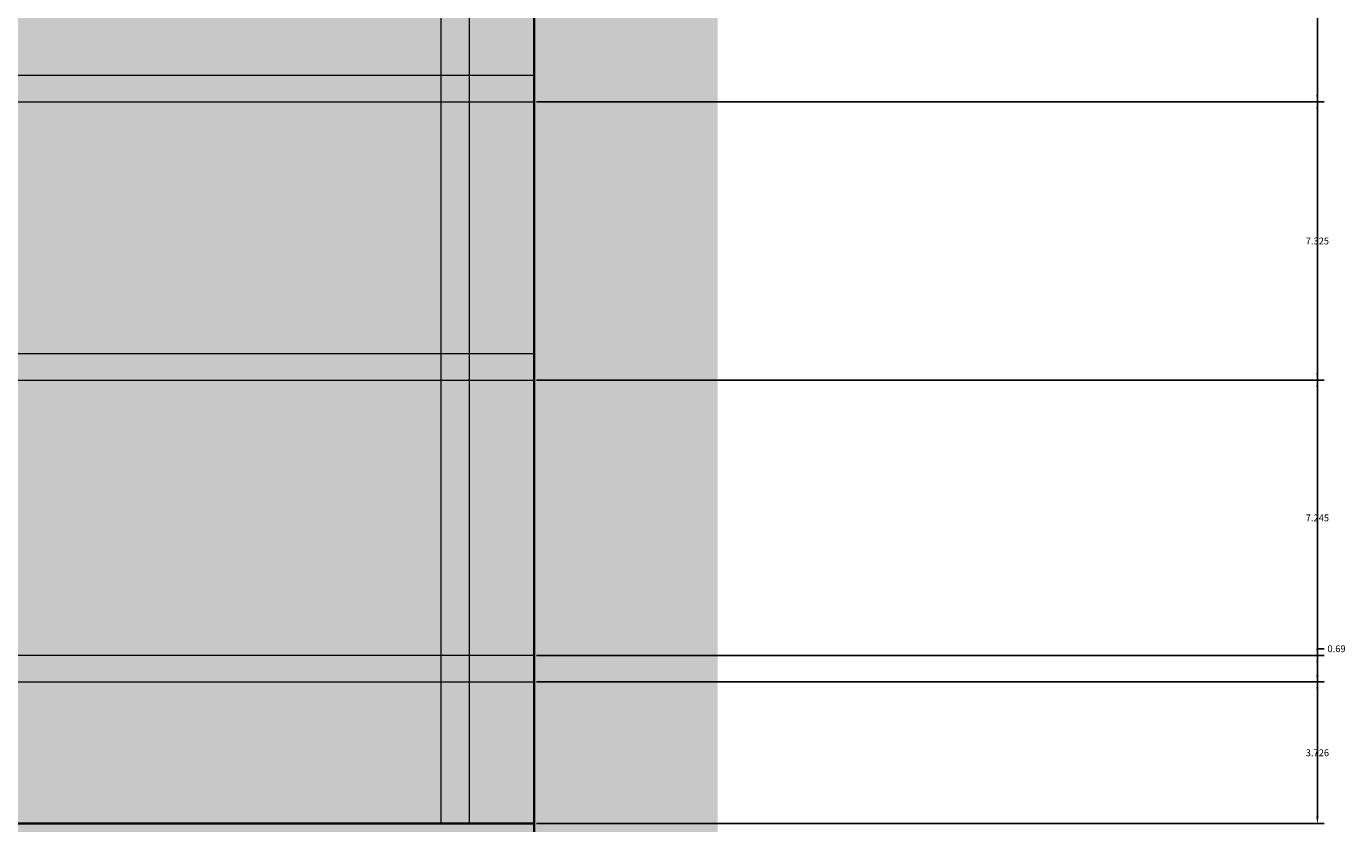
# Model space of a CAD drawing. Units: feet. Extents: x 2695 to 2912, y 795 to 1139.
# Tile 59 of 83: x 2877 to 2912, y 937 to 958. Entities that reach past the tile are written whole.
import ezdxf

# ---------------------------------------------------------------- set-up
doc = ezdxf.new("R2010")
doc.units = ezdxf.units.FT
for name, color, linetype, lineweight in [('A-ANNO-DIMS', 2, 'Continuous', 18), ('A-ELEV', 7, 'Continuous', 35), ('A-ELEV-PATT', 252, 'Continuous', 13), ('A-ELEV-RAIL', 8, 'Continuous', 18)]:
    doc.layers.add(name, color=color, linetype=linetype, lineweight=lineweight)
doc.styles.get("Standard").update_dxf_attribs({"font": 'arial.ttf'})
doc.dimstyles.get("Standard").update_dxf_attribs({"dimtxt": 0.18, "dimasz": 0.18, "dimexe": 0.18, "dimexo": 0.0625, "dimgap": 0.09, "dimtad": 0, "dimtih": 1, "dimtoh": 1, "dimdec": 1, "dimzin": 0, "dimdsep": 46, "dimlunit": 3, "dimtxsty": 'Standard', "dimcen": 0.09, "dimadec": 0, "dimazin": 0, "dimtfac": 1, "dimtdec": 1, "dimtofl": 0, "dimtmove": 0, "dimatfit": 3, "dimfxl": 1, "dimtolj": 1, "dimtzin": 0, "dimarcsym": 0})

# ---------------------------------------------------------------- blocks, each defined once
blk = doc.blocks.new('*D17')
at = {"layer": 'A-ANNO-DIMS', "color": 0, "lineweight": -2, "transparency": 16777216}
for p, q in [((2843.637, 1020.824), (2911.424, 1020.824)), ((2911.244, 1020.644), (2911.244, 979.059)), ((2911.244, 937.111), (2911.244, 978.695)), ((2890.699, 936.931), (2911.424, 936.931))]:
    blk.add_line(p, q, dxfattribs=at)
at = {"layer": 'A-ANNO-DIMS', "color": 0, "transparency": 16777216}
for points in [[(2911.214, 1020.644), (2911.274, 1020.644), (2911.244, 1020.824)], [(2911.214, 937.111), (2911.274, 937.111), (2911.244, 936.931)]]:
    blk.add_solid(points, dxfattribs=at)
at = {"layer": 'Defpoints', "color": 0, "transparency": 16777216}
for p in [(2843.575, 1020.824), (2911.244, 1020.824), (2890.636, 936.931)]:
    blk.add_point(p, dxfattribs=at)
at = {"layer": 'A-ANNO-DIMS', "color": 0, "transparency": 16777216, "insert": (2911.244, 978.877), "char_height": 0.18, "attachment_point": 5}
blk.add_mtext('\\A1;83.9', dxfattribs=at)
blk = doc.blocks.new('*D53')
at = {"layer": 'A-ANNO-DIMS', "color": 0, "lineweight": -2, "transparency": 16777216}
for p, q in [((2890.699, 940.657), (2911.424, 940.657)), ((2911.244, 940.477), (2911.244, 938.976)), ((2911.244, 937.111), (2911.244, 938.612)), ((2890.699, 936.931), (2911.424, 936.931))]:
    blk.add_line(p, q, dxfattribs=at)
at = {"layer": 'A-ANNO-DIMS', "color": 0, "transparency": 16777216}
for points in [[(2911.214, 940.477), (2911.274, 940.477), (2911.244, 940.657)], [(2911.214, 937.111), (2911.274, 937.111), (2911.244, 936.931)]]:
    blk.add_solid(points, dxfattribs=at)
at = {"layer": 'Defpoints', "color": 0, "transparency": 16777216}
for p in [(2890.636, 940.657), (2911.244, 940.657), (2890.636, 936.931)]:
    blk.add_point(p, dxfattribs=at)
at = {"layer": 'A-ANNO-DIMS', "color": 0, "transparency": 16777216, "insert": (2911.244, 938.794), "char_height": 0.18, "attachment_point": 5}
blk.add_mtext('\\A1;3.726', dxfattribs=at)
blk = doc.blocks.new('*D54')
at = {"layer": 'A-ANNO-DIMS', "color": 0, "lineweight": -2, "transparency": 16777216}
for p, q in [((2890.699, 941.351), (2911.424, 941.351)), ((2911.244, 941.351), (2911.244, 941.531)), ((2911.244, 941.531), (2911.424, 941.531)), ((2911.244, 940.837), (2911.244, 941.171)), ((2890.699, 940.657), (2911.424, 940.657))]:
    blk.add_line(p, q, dxfattribs=at)
at = {"layer": 'A-ANNO-DIMS', "color": 0, "transparency": 16777216}
for points in [[(2911.214, 941.171), (2911.274, 941.171), (2911.244, 941.351)], [(2911.214, 940.837), (2911.274, 940.837), (2911.244, 940.657)]]:
    blk.add_solid(points, dxfattribs=at)
at = {"layer": 'Defpoints', "color": 0, "transparency": 16777216}
for p in [(2890.636, 941.351), (2911.244, 941.351), (2890.636, 940.657)]:
    blk.add_point(p, dxfattribs=at)
at = {"layer": 'A-ANNO-DIMS', "color": 0, "transparency": 16777216, "insert": (2911.748, 941.531), "char_height": 0.18, "attachment_point": 5}
blk.add_mtext('\\A1;0.69', dxfattribs=at)
blk = doc.blocks.new('*D55')
at = {"layer": 'A-ANNO-DIMS', "color": 0, "lineweight": -2, "transparency": 16777216}
for p, q in [((2890.699, 948.595), (2911.424, 948.595)), ((2911.244, 948.415), (2911.244, 945.155)), ((2911.244, 941.531), (2911.244, 944.791)), ((2890.699, 941.351), (2911.424, 941.351))]:
    blk.add_line(p, q, dxfattribs=at)
at = {"layer": 'A-ANNO-DIMS', "color": 0, "transparency": 16777216}
for points in [[(2911.214, 948.415), (2911.274, 948.415), (2911.244, 948.595)], [(2911.214, 941.531), (2911.274, 941.531), (2911.244, 941.351)]]:
    blk.add_solid(points, dxfattribs=at)
at = {"layer": 'Defpoints', "color": 0, "transparency": 16777216}
for p in [(2890.636, 948.595), (2911.244, 948.595), (2890.636, 941.351)]:
    blk.add_point(p, dxfattribs=at)
at = {"layer": 'A-ANNO-DIMS', "color": 0, "transparency": 16777216, "insert": (2911.244, 944.973), "char_height": 0.18, "attachment_point": 5}
blk.add_mtext('\\A1;7.245', dxfattribs=at)
blk = doc.blocks.new('*D56')
at = {"layer": 'A-ANNO-DIMS', "color": 0, "lineweight": -2, "transparency": 16777216}
for p, q in [((2890.699, 955.92), (2911.424, 955.92)), ((2911.244, 955.74), (2911.244, 952.44)), ((2911.244, 948.775), (2911.244, 952.076)), ((2890.699, 948.595), (2911.424, 948.595))]:
    blk.add_line(p, q, dxfattribs=at)
at = {"layer": 'A-ANNO-DIMS', "color": 0, "transparency": 16777216}
for points in [[(2911.214, 955.74), (2911.274, 955.74), (2911.244, 955.92)], [(2911.214, 948.775), (2911.274, 948.775), (2911.244, 948.595)]]:
    blk.add_solid(points, dxfattribs=at)
at = {"layer": 'Defpoints', "color": 0, "transparency": 16777216}
for p in [(2890.636, 955.92), (2911.244, 955.92), (2890.636, 948.595)]:
    blk.add_point(p, dxfattribs=at)
at = {"layer": 'A-ANNO-DIMS', "color": 0, "transparency": 16777216, "insert": (2911.244, 952.258), "char_height": 0.18, "attachment_point": 5}
blk.add_mtext('\\A1;7.325', dxfattribs=at)
blk = doc.blocks.new('*D57')
at = {"layer": 'A-ANNO-DIMS', "color": 0, "lineweight": -2, "transparency": 16777216}
for p, q in [((2890.699, 964.133), (2911.424, 964.133)), ((2911.244, 963.953), (2911.244, 960.208)), ((2911.244, 956.1), (2911.244, 959.845)), ((2890.699, 955.92), (2911.424, 955.92))]:
    blk.add_line(p, q, dxfattribs=at)
at = {"layer": 'A-ANNO-DIMS', "color": 0, "transparency": 16777216}
for points in [[(2911.214, 963.953), (2911.274, 963.953), (2911.244, 964.133)], [(2911.214, 956.1), (2911.274, 956.1), (2911.244, 955.92)]]:
    blk.add_solid(points, dxfattribs=at)
at = {"layer": 'Defpoints', "color": 0, "transparency": 16777216}
for p in [(2890.636, 964.133), (2911.244, 964.133), (2890.636, 955.92)]:
    blk.add_point(p, dxfattribs=at)
at = {"layer": 'A-ANNO-DIMS', "color": 0, "transparency": 16777216, "insert": (2911.244, 960.027), "char_height": 0.18, "attachment_point": 5}
blk.add_mtext('\\A1;8.213', dxfattribs=at)

msp = doc.modelspace()

# ---------------------------------------------------------------- hatches: boundary and pattern name
at = {"layer": 'A-ELEV-PATT'}
h = msp.add_hatch(color=256, dxfattribs=at)
h.set_gradient(color1=(255, 255, 255), tint=1)
h.paths.add_polyline_path([(2770.6361, 1122.9306), (2710.6361, 1122.9306), (2710.6361, 1118.4096), (2770.6361, 1118.4096)])
h.paths.add_polyline_path([(2890.6361, 1107.8588), (2770.6361, 1107.8588), (2770.6361, 1103.3378), (2890.6361, 1103.3378)])
h.paths.add_polyline_path([(2890.6361, 1062.9306), (2710.6361, 1062.9306), (2710.6361, 1056.9306), (2710.6361, 936.9306), (2710.6361, 924.3105), (2716.5358, 924.3105), (2890.6361, 924.3105), (2890.6361, 936.9306), (2715.8852, 936.9306), (2715.8852, 1050.3105), (2890.6361, 1050.3105)])
h.paths.add_polyline_path([(2716.5358, 924.3105), (2710.6361, 924.3105), (2710.6361, 810.9306), (2716.5358, 810.9306)])
h = msp.add_hatch(color=256, dxfattribs=at)
h.set_gradient(color1=(147, 149, 152), color2=(147, 149, 152), tint=1)
h.paths.add_polyline_path([(2770.6361, 1118.4096), (2710.6361, 1118.4096), (2710.6361, 1062.9306), (2770.6361, 1062.9306)])
h.paths.add_polyline_path([(2890.6361, 1103.3378), (2770.6361, 1103.3378), (2770.6361, 1062.9306), (2890.6361, 1062.9306)])
h.paths.add_polyline_path([(2730.7081, 1048.1052), (2755.1125, 1048.1052), (2755.1125, 936.9306), (2770.6361, 936.9306), (2770.6361, 1050.3105), (2715.8852, 1050.3105), (2715.8852, 936.9306), (2730.7081, 936.9306)])
h.paths.add_polyline_path([(2890.6361, 1050.3105), (2770.6361, 1050.3105), (2770.6361, 971.9673), (2778.0341, 971.9673), (2778.0341, 1020.8235), (2843.575, 1020.8235), (2843.575, 971.9673), (2890.6361, 971.9673)])
h.paths.add_polyline_path([(2888.1882, 970.7156), (2843.575, 970.7156), (2843.575, 964.8267), (2888.1882, 964.8267)])
h.paths.add_polyline_path([(2888.1882, 964.1328), (2843.575, 964.1328), (2843.575, 956.614), (2888.1882, 956.614)])
h.paths.add_polyline_path([(2888.1882, 955.9202), (2843.575, 955.9202), (2843.575, 949.2892), (2888.1882, 949.2892)])
h.paths.add_polyline_path([(2888.1882, 948.5954), (2843.575, 948.5954), (2843.575, 941.3507), (2888.1882, 941.3507)])
h.paths.add_polyline_path([(2888.1882, 940.6569), (2843.575, 940.6569), (2843.575, 936.9306), (2888.1882, 936.9306)])
h.paths.add_polyline_path([(2890.6361, 970.7156), (2888.9368, 970.7156), (2888.9368, 964.8267), (2890.6361, 964.8267)])
h.paths.add_polyline_path([(2890.6361, 964.1328), (2888.9368, 964.1328), (2888.9368, 956.614), (2890.6361, 956.614)])
h.paths.add_polyline_path([(2890.6361, 955.9202), (2888.9368, 955.9202), (2888.9368, 949.2892), (2890.6361, 949.2892)])
h.paths.add_polyline_path([(2890.6361, 940.6569), (2888.9368, 940.6569), (2888.9368, 936.9306), (2890.6361, 936.9306)])
h.paths.add_polyline_path([(2890.6361, 948.5954), (2888.9368, 948.5954), (2888.9368, 941.3507), (2890.6361, 941.3507)])
h.paths.add_polyline_path([(2772.5216, 970.7156), (2770.6361, 970.7156), (2770.6361, 964.8267), (2772.5216, 964.8267)])
h.paths.add_polyline_path([(2772.5216, 964.1328), (2770.6361, 964.1328), (2770.6361, 956.614), (2772.5216, 956.614)])
h.paths.add_polyline_path([(2772.5216, 955.9202), (2770.6361, 955.9202), (2770.6361, 949.2892), (2772.5216, 949.2892)])
h.paths.add_polyline_path([(2772.5216, 948.5954), (2770.6361, 948.5954), (2770.6361, 941.3507), (2772.5216, 941.3507)])
h.paths.add_polyline_path([(2772.5216, 940.6569), (2770.6361, 940.6569), (2770.6361, 936.9306), (2772.5216, 936.9306)])
h.paths.add_polyline_path([(2778.0341, 940.6569), (2773.2702, 940.6569), (2773.2702, 936.9306), (2778.0341, 936.9306)])
h.paths.add_polyline_path([(2778.0341, 970.7156), (2773.2702, 970.7156), (2773.2702, 964.8267), (2778.0341, 964.8267)])
h.paths.add_polyline_path([(2778.0341, 964.1328), (2773.2702, 964.1328), (2773.2702, 956.614), (2778.0341, 956.614)])
h.paths.add_polyline_path([(2778.0341, 955.9202), (2773.2702, 955.9202), (2773.2702, 949.2892), (2778.0341, 949.2892)])
h.paths.add_polyline_path([(2778.0341, 948.5954), (2773.2702, 948.5954), (2773.2702, 941.3507), (2778.0341, 941.3507)])
h.paths.add_polyline_path([(2810.0407, 940.6569), (2780.0341, 940.6569), (2780.0341, 936.9306), (2810.0407, 936.9306)])
h.paths.add_polyline_path([(2890.6361, 924.3105), (2770.6361, 924.3105), (2770.6361, 810.9306), (2773.5029, 810.9306), (2773.5029, 905.5143), (2805.9398, 905.5143), (2838.3767, 905.5143), (2838.3767, 810.9306), (2890.6361, 810.9306)])
h = msp.add_hatch(color=256, dxfattribs=at)
h.set_gradient(color1=(255, 255, 255), tint=1)
h.paths.add_polyline_path([(2895.4694, 1107.8588), (2890.6361, 1107.8588), (2890.6361, 810.9306), (2895.4694, 810.9306)])
h = msp.add_hatch(color=256, dxfattribs=at)
h.set_gradient(color1=(255, 255, 255), tint=1)
h.paths.add_polyline_path([(2890.6361, 1050.3105), (2881.9484, 1050.3105), (2881.9484, 971.9673), (2890.6361, 971.9673)])
h.paths.add_polyline_path([(2888.1882, 970.7156), (2881.9484, 970.7156), (2881.9484, 964.8267), (2888.1882, 964.8267)])
h.paths.add_polyline_path([(2890.6361, 970.7156), (2888.9368, 970.7156), (2888.9368, 964.8267), (2890.6361, 964.8267)])
h.paths.add_polyline_path([(2888.1882, 964.1328), (2881.9484, 964.1328), (2881.9484, 956.614), (2888.1882, 956.614)])
h.paths.add_polyline_path([(2890.6361, 964.1328), (2888.9368, 964.1328), (2888.9368, 956.614), (2890.6361, 956.614)])
h.paths.add_polyline_path([(2888.1882, 955.9202), (2881.9484, 955.9202), (2881.9484, 949.2892), (2888.1882, 949.2892)])
h.paths.add_polyline_path([(2890.6361, 955.9202), (2888.9368, 955.9202), (2888.9368, 949.2892), (2890.6361, 949.2892)])
h.paths.add_polyline_path([(2888.1882, 948.5954), (2881.9484, 948.5954), (2881.9484, 941.3507), (2888.1882, 941.3507)])
h.paths.add_polyline_path([(2890.6361, 948.5954), (2888.9368, 948.5954), (2888.9368, 941.3507), (2890.6361, 941.3507)])
h.paths.add_polyline_path([(2888.1882, 940.6569), (2881.9484, 940.6569), (2881.9484, 936.9306), (2888.1882, 936.9306)])
h = msp.add_hatch(color=256, dxfattribs=at)
h.set_gradient(color2=(0, 0, 0), tint=1)
h.paths.add_polyline_path([(2772.5216, 971.9673), (2770.6361, 971.9673), (2770.6361, 970.7156), (2772.5216, 970.7156)])
h.paths.add_polyline_path([(2773.2702, 971.9673), (2772.5216, 971.9673), (2772.5216, 970.7156), (2773.2702, 970.7156)])
h.paths.add_polyline_path([(2778.0341, 971.9673), (2773.2702, 971.9673), (2773.2702, 970.7156), (2778.0341, 970.7156)])
h.paths.add_polyline_path([(2780.0341, 971.9673), (2778.0341, 971.9673), (2778.0341, 970.7156), (2780.0341, 970.7156)])
h.paths.add_polyline_path([(2841.575, 971.9673), (2780.0341, 971.9673), (2780.0341, 970.7156), (2841.575, 970.7156)])
h.paths.add_polyline_path([(2843.575, 971.9673), (2841.575, 971.9673), (2841.575, 970.7156), (2843.575, 970.7156)])
h.paths.add_polyline_path([(2888.1882, 971.9673), (2843.575, 971.9673), (2843.575, 970.7156), (2888.1882, 970.7156)])
h.paths.add_polyline_path([(2888.9368, 971.9673), (2888.1882, 971.9673), (2888.1882, 970.7156), (2888.9368, 970.7156)], flags=17)
h.paths.add_polyline_path([(2890.6361, 971.9673), (2888.9368, 971.9673), (2888.9368, 970.7156), (2890.6361, 970.7156)])
h.paths.add_polyline_path([(2888.9368, 971.9673), (2888.1882, 971.9673), (2888.1882, 964.8267), (2888.9368, 964.8267)])
h.paths.add_polyline_path([(2888.9368, 964.8267), (2888.1882, 964.8267), (2888.1882, 964.1328), (2888.9368, 964.1328)])
h.paths.add_polyline_path([(2890.6361, 964.8267), (2888.9368, 964.8267), (2888.9368, 964.1328), (2890.6361, 964.1328)])
h.paths.add_polyline_path([(2888.1882, 964.8267), (2770.6361, 964.8267), (2770.6361, 964.1328), (2888.1882, 964.1328)])
h.paths.add_polyline_path([(2888.9368, 964.1328), (2888.1882, 964.1328), (2888.1882, 936.9306), (2888.9368, 936.9306)])
h.paths.add_polyline_path([(2890.6361, 956.614), (2888.9368, 956.614), (2888.9368, 955.9202), (2890.6361, 955.9202)])
h.paths.add_polyline_path([(2888.1882, 956.614), (2770.6361, 956.614), (2770.6361, 955.9202), (2888.1882, 955.9202)])
h.paths.add_polyline_path([(2890.6361, 949.2892), (2888.9368, 949.2892), (2888.9368, 948.5954), (2890.6361, 948.5954)])
h.paths.add_polyline_path([(2888.1882, 949.2892), (2770.6361, 949.2892), (2770.6361, 948.5954), (2888.1882, 948.5954)])
h.paths.add_polyline_path([(2890.6361, 941.3507), (2888.9368, 941.3507), (2888.9368, 940.6569), (2890.6361, 940.6569)])
h.paths.add_polyline_path([(2888.1882, 941.3507), (2770.6361, 941.3507), (2770.6361, 940.6569), (2888.1882, 940.6569)])
h.paths.add_polyline_path([(2773.2702, 970.7156), (2772.5216, 970.7156), (2772.5216, 964.8267), (2773.2702, 964.8267)])
h.paths.add_polyline_path([(2773.2702, 964.1328), (2772.5216, 964.1328), (2772.5216, 956.614), (2773.2702, 956.614)])
h.paths.add_polyline_path([(2773.2702, 955.9202), (2772.5216, 955.9202), (2772.5216, 936.9306), (2773.2702, 936.9306)])
h.paths.add_polyline_path([(2810.7893, 970.7156), (2810.0407, 970.7156), (2810.0407, 964.8267), (2810.7893, 964.8267)], flags=17)
h.paths.add_polyline_path([(2810.7893, 964.1328), (2810.0407, 964.1328), (2810.0407, 956.614), (2810.7893, 956.614)], flags=17)
h.paths.add_polyline_path([(2810.7893, 955.9202), (2810.0407, 955.9202), (2810.0407, 949.2892), (2810.7893, 949.2892)], flags=17)
h.paths.add_polyline_path([(2810.7893, 971.9673), (2810.0407, 971.9673), (2810.0407, 941.3507), (2810.7893, 941.3507)])
h.paths.add_polyline_path([(2810.7893, 940.6569), (2810.0407, 940.6569), (2810.0407, 936.9306), (2810.7893, 936.9306)])
h.paths.add_polyline_path([(2780.0341, 1018.8235), (2841.575, 1018.8235), (2841.575, 971.9673), (2843.575, 971.9673), (2843.575, 1020.8235), (2778.0341, 1020.8235), (2778.0341, 971.9673), (2780.0341, 971.9673)])
h.paths.add_polyline_path([(2780.0341, 970.7156), (2778.0341, 970.7156), (2778.0341, 964.8267), (2780.0341, 964.8267)])
h.paths.add_polyline_path([(2780.0341, 964.1328), (2778.0341, 964.1328), (2778.0341, 956.614), (2780.0341, 956.614)])
h.paths.add_polyline_path([(2780.0341, 955.9202), (2778.0341, 955.9202), (2778.0341, 949.2892), (2780.0341, 949.2892)])
h.paths.add_polyline_path([(2780.0341, 948.5954), (2778.0341, 948.5954), (2778.0341, 941.3507), (2780.0341, 941.3507)])
h.paths.add_polyline_path([(2780.0341, 940.6569), (2778.0341, 940.6569), (2778.0341, 936.9306), (2780.0341, 936.9306)])
h.paths.add_polyline_path([(2843.575, 940.6569), (2841.575, 940.6569), (2841.575, 936.9306), (2843.575, 936.9306)])
h.paths.add_polyline_path([(2843.575, 948.5954), (2841.575, 948.5954), (2841.575, 941.3507), (2843.575, 941.3507)])
h.paths.add_polyline_path([(2843.575, 970.7156), (2841.575, 970.7156), (2841.575, 964.8267), (2843.575, 964.8267)])
h.paths.add_polyline_path([(2843.575, 964.1328), (2841.575, 964.1328), (2841.575, 956.614), (2843.575, 956.614)])
h.paths.add_polyline_path([(2843.575, 955.9202), (2841.575, 955.9202), (2841.575, 949.2892), (2843.575, 949.2892)])
h.paths.add_polyline_path([(2805.0538, 874.1057), (2803.9681, 874.1057), (2803.9681, 846.2857), (2805.0538, 846.2857)])
h.paths.add_polyline_path([(2758.1515, 902.577), (2724.1893, 902.577), (2724.1893, 874.8571), (2758.1515, 874.8571)])
h.paths.add_polyline_path([(2726.1893, 900.577), (2756.1515, 900.577), (2756.1515, 876.8571), (2726.1893, 876.8571)], flags=16)
h.paths.add_polyline_path([(2740.7302, 900.577), (2741.6105, 900.577), (2741.6105, 876.8571), (2740.7302, 876.8571)], flags=0)

# ---------------------------------------------------------------- linework, layer by layer
at = {"layer": 'A-ELEV'}
for p, q in [((2890.6361, 810.9306), (2890.6361, 1107.8588)), ((2890.6361, 1062.9306), (2890.6361, 810.9306)), ((2715.8852, 936.9306), (2890.6361, 936.9306)), ((2715.8852, 936.9306), (2890.6361, 936.9306))]:
    msp.add_line(p, q, dxfattribs=at)
msp.add_lwpolyline([(2890.6361, 936.9306), (2890.6361, 924.3105), (2710.6361, 924.3105), (2710.6361, 936.9306)], dxfattribs=at)
at = {"layer": 'A-ELEV-RAIL'}
for points in [[(2888.9368, 971.9673), (2888.1882, 971.9673), (2888.1882, 936.9306), (2888.9368, 936.9306)], [(2770.6361, 955.9202), (2890.6361, 955.9202), (2890.6361, 956.614), (2770.6361, 956.614)], [(2770.6361, 948.5954), (2890.6361, 948.5954), (2890.6361, 949.2892), (2770.6361, 949.2892)], [(2770.6361, 940.6569), (2890.6361, 940.6569), (2890.6361, 941.3507), (2770.6361, 941.3507)]]:
    msp.add_lwpolyline(points, close=True, dxfattribs=at)

# ---------------------------------------------------------------- dimensions: what is measured, and where the dimension line sits
at = {"layer": 'A-ANNO-DIMS'}
for base, p1, p2, override, picture, middle in [((2911.2444, 1020.8235), (2890.6361, 936.9306), (2843.575, 1020.8235), {"dimdec": 1, "dimlfac": 1, "dimrnd": 0, "dimzin": 0, "dimdsep": 46, "dimlunit": 2}, '*D17', (2911.2444, 978.877)), ((2911.2444, 964.1328), (2890.6361, 955.9202), (2890.6361, 964.1328), {"dimdec": 3, "dimlfac": 1, "dimrnd": 0, "dimzin": 0, "dimdsep": 46, "dimlunit": 2}, '*D57', (2911.2444, 960.0265)), ((2911.2444, 955.9202), (2890.6361, 948.5954), (2890.6361, 955.9202), {"dimdec": 3, "dimlfac": 1, "dimrnd": 0, "dimzin": 0, "dimdsep": 46, "dimlunit": 2}, '*D56', (2911.2444, 952.2578)), ((2911.2444, 948.5954), (2890.6361, 941.3507), (2890.6361, 948.5954), {"dimdec": 3, "dimlfac": 1, "dimrnd": 0, "dimzin": 0, "dimdsep": 46, "dimlunit": 2}, '*D55', (2911.2444, 944.973)), ((2911.2444, 941.3507), (2890.6361, 940.6569), (2890.6361, 941.3507), {"dimdec": 2, "dimlfac": 1, "dimrnd": 0, "dimzin": 0, "dimdsep": 46, "dimlunit": 2}, '*D54', (2911.7483, 941.5307)), ((2911.2444, 940.6569), (2890.6361, 936.9306), (2890.6361, 940.6569), {"dimdec": 3, "dimlfac": 1, "dimrnd": 0, "dimzin": 0, "dimdsep": 46, "dimlunit": 2}, '*D53', (2911.2444, 938.7937))]:
    dim = msp.add_linear_dim(base=base, p1=p1, p2=p2, angle=90, dimstyle='Standard', override=override, dxfattribs=at)
    dim.commit()
    dim.dimension.update_dxf_attribs({"geometry": picture, "text_midpoint": middle})

doc.saveas('drawing.dxf')
